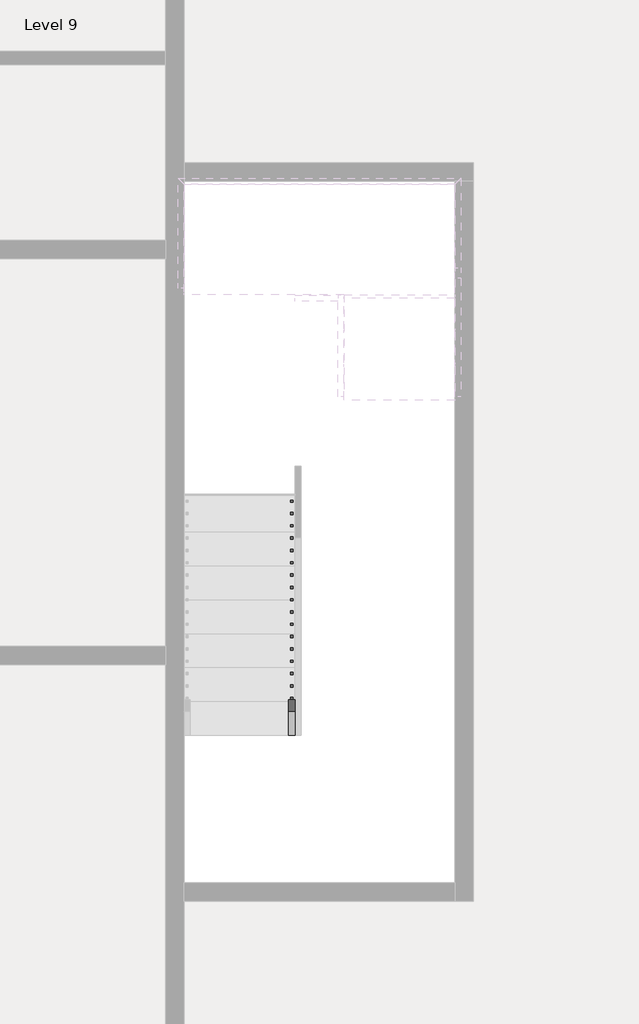
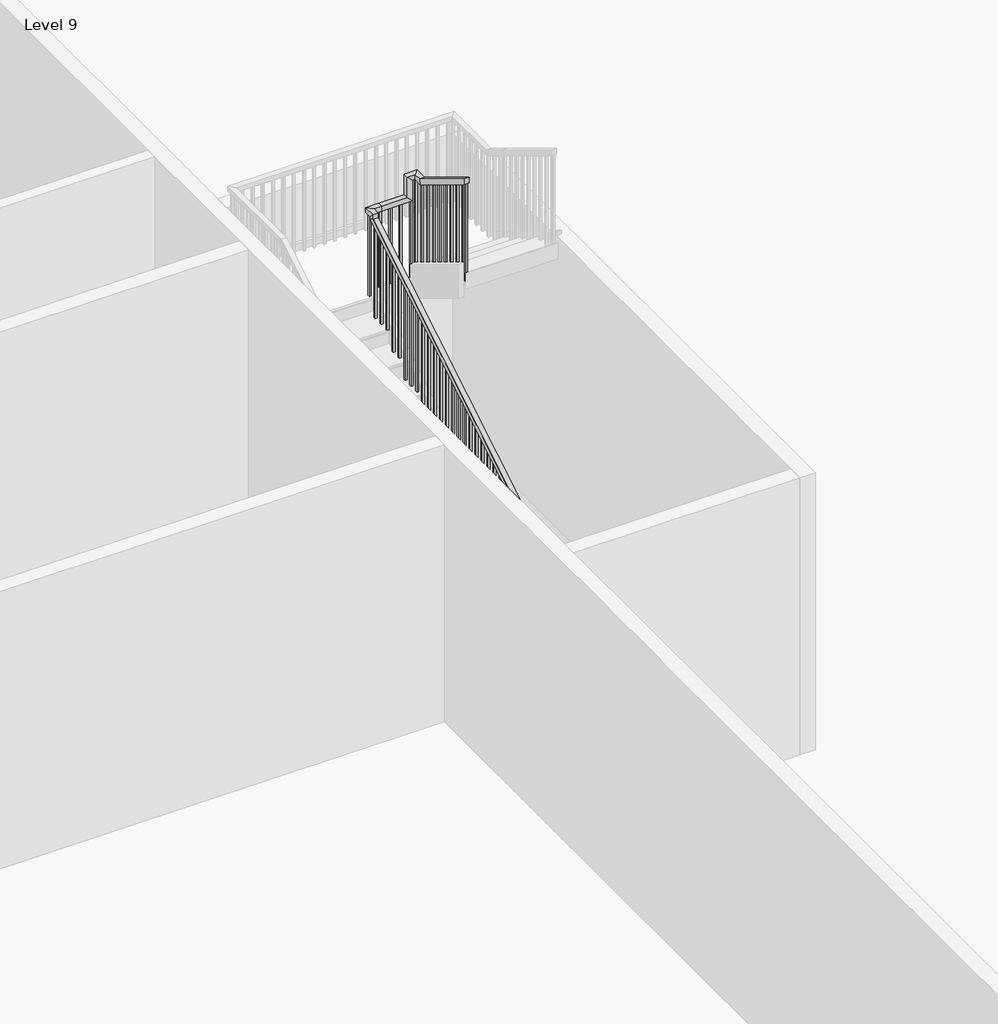
# One storey, part 5 of 8: 1 railing.
"""IFC4 building model written with IfcOpenShell, lengths in millimetres."""

from ifc_helpers import new_model, si_unit, frame, origin, place, context, project, spatial, polyline, outline, extrude, faceted_brep, element, save

model = new_model("IFC4")

# Units and contexts
model_context = context("Model", 3, world=origin())
ifc_project = project(units=[si_unit("LENGTHUNIT", "METRE", prefix="MILLI")], contexts=[model_context])

# Site, building, storey
site = spatial("IfcSite", under=ifc_project)
building = spatial("IfcBuilding", under=site)
storey = spatial("IfcBuildingStorey", under=building, Name="Level 9", Elevation=49618.6172466)

# Railing
placement = place(None, origin())
element("IfcRailing", 1, ObjectType="Handrail - Rectangular", at=placement, inside=storey, context=model_context, shape_type="SolidModel", body=[
    faceted_brep([(-2753.8415084, -23154.3851539, 50702.3505799), (-2753.8415084, -23154.3851539, 50642.9491197), (-2703.0415084, -23154.3851539, 50642.9491197), (-2703.0415084, -23154.3851539, 50702.3505799), (-2753.8415084, -19598.3851539, 52857.5020951), (-2753.8415084, -19547.5851539, 52828.8885136), (-2703.0415084, -19547.5851539, 52828.8885136), (-2703.0415084, -19598.3851539, 52857.5020951), (-2753.8415084, -19598.3851539, 52903.6839133), (-2753.8415084, -19547.5851539, 52852.8839133), (-2703.0415084, -19547.5851539, 52852.8839133), (-2703.0415084, -19598.3851539, 52903.6839133), (-2753.8415084, -19471.3851539, 52903.6839133), (-2753.8415084, -19471.3851539, 52852.8839133), (-2703.0415084, -19522.1851539, 52852.8839133), (-2703.0415084, -19522.1851539, 52903.6839133), (-2626.8415084, -19471.3851539, 52903.6839133), (-2626.8415084, -19471.3851539, 52852.8839133), (-2626.8415084, -19522.1851539, 52852.8839133), (-2626.8415084, -19522.1851539, 52903.6839133), (-2372.8415084, -19471.3851539, 52903.6839133), (-2322.0415084, -19471.3851539, 52852.8839133), (-2322.0415084, -19522.1851539, 52852.8839133), (-2372.8415084, -19522.1851539, 52903.6839133), (-2372.8415084, -19471.3851539, 53119.1990648), (-2322.0415084, -19471.3851539, 53068.3990648), (-2322.0415084, -19522.1851539, 53068.3990648), (-2372.8415084, -19522.1851539, 53119.1990648), (-2245.8415084, -19471.3851539, 53119.1990648), (-2245.8415084, -19471.3851539, 53068.3990648), (-2296.6415084, -19522.1851539, 53068.3990648), (-2296.6415084, -19522.1851539, 53119.1990648), (-2245.8415084, -19598.3851539, 53119.1990648), (-2245.8415084, -19612.5775633, 53068.3990648), (-2296.6415084, -19612.5775633, 53068.3990648), (-2296.6415084, -19598.3851539, 53119.1990648), (-2245.8415084, -20360.3851539, 53581.0172466), (-2296.6415084, -20360.3851539, 53581.0172466), (-2296.6415084, -20360.3851539, 53521.6157863), (-2245.8415084, -20360.3851539, 53521.6157863)], [[[0, 1, 2, 3]], [[1, 0, 4, 5]], [[2, 1, 5, 6]], [[3, 2, 6, 7]], [[0, 3, 7, 4]], [[5, 4, 8, 9]], [[6, 5, 9, 10]], [[7, 6, 10, 11]], [[4, 7, 11, 8]], [[9, 8, 12, 13]], [[10, 9, 13, 14]], [[11, 10, 14, 15]], [[8, 11, 15, 12]], [[13, 12, 16, 17]], [[14, 13, 17, 18]], [[15, 14, 18, 19]], [[12, 15, 19, 16]], [[17, 16, 20, 21]], [[18, 17, 21, 22]], [[19, 18, 22, 23]], [[16, 19, 23, 20]], [[21, 20, 24, 25]], [[22, 21, 25, 26]], [[23, 22, 26, 27]], [[20, 23, 27, 24]], [[25, 24, 28, 29]], [[26, 25, 29, 30]], [[27, 26, 30, 31]], [[24, 27, 31, 28]], [[29, 28, 32, 33]], [[30, 29, 33, 34]], [[31, 30, 34, 35]], [[28, 31, 35, 32]], [[36, 37, 38, 39]], [[33, 32, 36, 39]], [[34, 33, 39, 38]], [[35, 34, 38, 37]], [[32, 35, 37, 36]]]),
    extrude(outline(polyline([(-20319.1101539, 53496.6006348), (-20300.0601539, 53485.0551803), (-20300.0601539, 52497.2839133), (-20319.1101539, 52497.2839133), (-20319.1101539, 53496.6006348)])), frame((-2280.7665084, 0.0, 0.0), z_axis=(1.0, 0.0, 0.0), x_axis=(0.0, 1.0, 0.0)), (0.0, 0.0, 1.0), 19.05),
    extrude(outline(polyline([(-20217.5101539, 53435.0248773), (-20198.4601539, 53423.4794227), (-20198.4601539, 52497.2839133), (-20217.5101539, 52497.2839133), (-20217.5101539, 53435.0248773)])), frame((-2280.7665084, 0.0, 0.0), z_axis=(1.0, 0.0, 0.0), x_axis=(0.0, 1.0, 0.0)), (0.0, 0.0, 1.0), 19.05),
    extrude(outline(polyline([(-20115.9101539, 53373.4491197), (-20096.8601539, 53361.9036651), (-20096.8601539, 52497.2839133), (-20115.9101539, 52497.2839133), (-20115.9101539, 53373.4491197)])), frame((-2280.7665084, 0.0, 0.0), z_axis=(1.0, 0.0, 0.0), x_axis=(0.0, 1.0, 0.0)), (0.0, 0.0, 1.0), 19.05),
    extrude(outline(polyline([(-20014.3101539, 53311.8733621), (-19995.2601539, 53300.3279076), (-19995.2601539, 52327.9505799), (-20014.3101539, 52327.9505799), (-20014.3101539, 53311.8733621)])), frame((-2280.7665084, 0.0, 0.0), z_axis=(1.0, 0.0, 0.0), x_axis=(0.0, 1.0, 0.0)), (0.0, 0.0, 1.0), 19.05),
    extrude(outline(polyline([(-19912.7101539, 53250.2976045), (-19893.6601539, 53238.75215), (-19893.6601539, 52327.9505799), (-19912.7101539, 52327.9505799), (-19912.7101539, 53250.2976045)])), frame((-2280.7665084, 0.0, 0.0), z_axis=(1.0, 0.0, 0.0), x_axis=(0.0, 1.0, 0.0)), (0.0, 0.0, 1.0), 19.05),
    extrude(outline(polyline([(-19811.1101539, 53188.721847), (-19792.0601539, 53177.1763924), (-19792.0601539, 52327.9505799), (-19811.1101539, 52327.9505799), (-19811.1101539, 53188.721847)])), frame((-2280.7665084, 0.0, 0.0), z_axis=(1.0, 0.0, 0.0), x_axis=(0.0, 1.0, 0.0)), (0.0, 0.0, 1.0), 19.05),
    extrude(outline(polyline([(-19709.5101539, 53127.1460894), (-19690.4601539, 53115.6006348), (-19690.4601539, 52158.6172466), (-19709.5101539, 52158.6172466), (-19709.5101539, 53127.1460894)])), frame((-2280.7665084, 0.0, 0.0), z_axis=(1.0, 0.0, 0.0), x_axis=(0.0, 1.0, 0.0)), (0.0, 0.0, 1.0), 19.05),
    extrude(outline(polyline([(-19607.9101539, 53065.5703318), (-19588.8601539, 53054.0248773), (-19588.8601539, 52158.6172466), (-19607.9101539, 52158.6172466), (-19607.9101539, 53065.5703318)])), frame((-2280.7665084, 0.0, 0.0), z_axis=(1.0, 0.0, 0.0), x_axis=(0.0, 1.0, 0.0)), (0.0, 0.0, 1.0), 19.05),
    extrude(outline(polyline([(-2331.5665084, -19506.3101539), (-2331.5665084, -19487.2601539), (-2312.5165084, -19487.2601539), (-2312.5165084, -19506.3101539), (-2331.5665084, -19506.3101539)])), frame((0.0, 0.0, 51989.2839133), z_axis=(0.0, 0.0, 1.0), x_axis=(1.0, 0.0, 0.0)), (0.0, 0.0, 1.0), 1079.1151515),
    extrude(outline(polyline([(-2433.1665084, -19506.3101539), (-2433.1665084, -19487.2601539), (-2414.1165084, -19487.2601539), (-2414.1165084, -19506.3101539), (-2433.1665084, -19506.3101539)])), frame((0.0, 0.0, 51989.2839133), z_axis=(0.0, 0.0, 1.0), x_axis=(1.0, 0.0, 0.0)), (0.0, 0.0, 1.0), 863.6),
    extrude(outline(polyline([(-2534.7665084, -19506.3101539), (-2534.7665084, -19487.2601539), (-2515.7165084, -19487.2601539), (-2515.7165084, -19506.3101539), (-2534.7665084, -19506.3101539)])), frame((0.0, 0.0, 51989.2839133), z_axis=(0.0, 0.0, 1.0), x_axis=(1.0, 0.0, 0.0)), (0.0, 0.0, 1.0), 863.6),
    extrude(outline(polyline([(-2636.3665084, -19506.3101539), (-2636.3665084, -19487.2601539), (-2617.3165084, -19487.2601539), (-2617.3165084, -19506.3101539), (-2636.3665084, -19506.3101539)])), frame((0.0, 0.0, 51989.2839133), z_axis=(0.0, 0.0, 1.0), x_axis=(1.0, 0.0, 0.0)), (0.0, 0.0, 1.0), 863.6),
    extrude(outline(polyline([(-19607.9101539, 52792.3279076), (-19588.8601539, 52803.8733621), (-19588.8601539, 51819.9505799), (-19607.9101539, 51819.9505799), (-19607.9101539, 52792.3279076)])), frame((-2737.9665084, 0.0, 0.0), z_axis=(1.0, 0.0, 0.0), x_axis=(0.0, 1.0, 0.0)), (0.0, 0.0, 1.0), 19.05),
    extrude(outline(polyline([(-19709.5101539, 52730.75215), (-19690.4601539, 52742.2976045), (-19690.4601539, 51819.9505799), (-19709.5101539, 51819.9505799), (-19709.5101539, 52730.75215)])), frame((-2737.9665084, 0.0, 0.0), z_axis=(1.0, 0.0, 0.0), x_axis=(0.0, 1.0, 0.0)), (0.0, 0.0, 1.0), 19.05),
    extrude(outline(polyline([(-19811.1101539, 52669.1763924), (-19792.0601539, 52680.721847), (-19792.0601539, 51819.9505799), (-19811.1101539, 51819.9505799), (-19811.1101539, 52669.1763924)])), frame((-2737.9665084, 0.0, 0.0), z_axis=(1.0, 0.0, 0.0), x_axis=(0.0, 1.0, 0.0)), (0.0, 0.0, 1.0), 19.05),
    extrude(outline(polyline([(-19912.7101539, 52607.6006348), (-19893.6601539, 52619.1460894), (-19893.6601539, 51650.6172466), (-19912.7101539, 51650.6172466), (-19912.7101539, 52607.6006348)])), frame((-2737.9665084, 0.0, 0.0), z_axis=(1.0, 0.0, 0.0), x_axis=(0.0, 1.0, 0.0)), (0.0, 0.0, 1.0), 19.05),
    extrude(outline(polyline([(-20014.3101539, 52546.0248773), (-19995.2601539, 52557.5703318), (-19995.2601539, 51650.6172466), (-20014.3101539, 51650.6172466), (-20014.3101539, 52546.0248773)])), frame((-2737.9665084, 0.0, 0.0), z_axis=(1.0, 0.0, 0.0), x_axis=(0.0, 1.0, 0.0)), (0.0, 0.0, 1.0), 19.05),
    extrude(outline(polyline([(-20115.9101539, 52484.4491197), (-20096.8601539, 52495.9945742), (-20096.8601539, 51481.2839133), (-20115.9101539, 51481.2839133), (-20115.9101539, 52484.4491197)])), frame((-2737.9665084, 0.0, 0.0), z_axis=(1.0, 0.0, 0.0), x_axis=(0.0, 1.0, 0.0)), (0.0, 0.0, 1.0), 19.05),
    extrude(outline(polyline([(-20217.5101539, 52422.8733621), (-20198.4601539, 52434.4188166), (-20198.4601539, 51481.2839133), (-20217.5101539, 51481.2839133), (-20217.5101539, 52422.8733621)])), frame((-2737.9665084, 0.0, 0.0), z_axis=(1.0, 0.0, 0.0), x_axis=(0.0, 1.0, 0.0)), (0.0, 0.0, 1.0), 19.05),
    extrude(outline(polyline([(-20319.1101539, 52361.2976045), (-20300.0601539, 52372.8430591), (-20300.0601539, 51481.2839133), (-20319.1101539, 51481.2839133), (-20319.1101539, 52361.2976045)])), frame((-2737.9665084, 0.0, 0.0), z_axis=(1.0, 0.0, 0.0), x_axis=(0.0, 1.0, 0.0)), (0.0, 0.0, 1.0), 19.05),
    extrude(outline(polyline([(-20420.7101539, 52299.721847), (-20401.6601539, 52311.2673015), (-20401.6601539, 51311.9505799), (-20420.7101539, 51311.9505799), (-20420.7101539, 52299.721847)])), frame((-2737.9665084, 0.0, 0.0), z_axis=(1.0, 0.0, 0.0), x_axis=(0.0, 1.0, 0.0)), (0.0, 0.0, 1.0), 19.05),
    extrude(outline(polyline([(-20522.3101539, 52238.1460894), (-20503.2601539, 52249.6915439), (-20503.2601539, 51311.9505799), (-20522.3101539, 51311.9505799), (-20522.3101539, 52238.1460894)])), frame((-2737.9665084, 0.0, 0.0), z_axis=(1.0, 0.0, 0.0), x_axis=(0.0, 1.0, 0.0)), (0.0, 0.0, 1.0), 19.05),
    extrude(outline(polyline([(-20623.9101539, 52176.5703318), (-20604.8601539, 52188.1157863), (-20604.8601539, 51311.9505799), (-20623.9101539, 51311.9505799), (-20623.9101539, 52176.5703318)])), frame((-2737.9665084, 0.0, 0.0), z_axis=(1.0, 0.0, 0.0), x_axis=(0.0, 1.0, 0.0)), (0.0, 0.0, 1.0), 19.05),
    extrude(outline(polyline([(-20725.5101539, 52114.9945742), (-20706.4601539, 52126.5400288), (-20706.4601539, 51142.6172466), (-20725.5101539, 51142.6172466), (-20725.5101539, 52114.9945742)])), frame((-2737.9665084, 0.0, 0.0), z_axis=(1.0, 0.0, 0.0), x_axis=(0.0, 1.0, 0.0)), (0.0, 0.0, 1.0), 19.05),
    extrude(outline(polyline([(-20827.1101539, 52053.4188166), (-20808.0601539, 52064.9642712), (-20808.0601539, 51142.6172466), (-20827.1101539, 51142.6172466), (-20827.1101539, 52053.4188166)])), frame((-2737.9665084, 0.0, 0.0), z_axis=(1.0, 0.0, 0.0), x_axis=(0.0, 1.0, 0.0)), (0.0, 0.0, 1.0), 19.05),
    extrude(outline(polyline([(-20928.7101539, 51991.8430591), (-20909.6601539, 52003.3885136), (-20909.6601539, 51142.6172466), (-20928.7101539, 51142.6172466), (-20928.7101539, 51991.8430591)])), frame((-2737.9665084, 0.0, 0.0), z_axis=(1.0, 0.0, 0.0), x_axis=(0.0, 1.0, 0.0)), (0.0, 0.0, 1.0), 19.05),
    extrude(outline(polyline([(-21030.3101539, 51930.2673015), (-21011.2601539, 51941.812756), (-21011.2601539, 50973.2839133), (-21030.3101539, 50973.2839133), (-21030.3101539, 51930.2673015)])), frame((-2737.9665084, 0.0, 0.0), z_axis=(1.0, 0.0, 0.0), x_axis=(0.0, 1.0, 0.0)), (0.0, 0.0, 1.0), 19.05),
    extrude(outline(polyline([(-21131.9101539, 51868.6915439), (-21112.8601539, 51880.2369985), (-21112.8601539, 50973.2839133), (-21131.9101539, 50973.2839133), (-21131.9101539, 51868.6915439)])), frame((-2737.9665084, 0.0, 0.0), z_axis=(1.0, 0.0, 0.0), x_axis=(0.0, 1.0, 0.0)), (0.0, 0.0, 1.0), 19.05),
    extrude(outline(polyline([(-21233.5101539, 51807.1157863), (-21214.4601539, 51818.6612409), (-21214.4601539, 50803.9505799), (-21233.5101539, 50803.9505799), (-21233.5101539, 51807.1157863)])), frame((-2737.9665084, 0.0, 0.0), z_axis=(1.0, 0.0, 0.0), x_axis=(0.0, 1.0, 0.0)), (0.0, 0.0, 1.0), 19.05),
    extrude(outline(polyline([(-21335.1101539, 51745.5400288), (-21316.0601539, 51757.0854833), (-21316.0601539, 50803.9505799), (-21335.1101539, 50803.9505799), (-21335.1101539, 51745.5400288)])), frame((-2737.9665084, 0.0, 0.0), z_axis=(1.0, 0.0, 0.0), x_axis=(0.0, 1.0, 0.0)), (0.0, 0.0, 1.0), 19.05),
    extrude(outline(polyline([(-21436.7101539, 51683.9642712), (-21417.6601539, 51695.5097257), (-21417.6601539, 50803.9505799), (-21436.7101539, 50803.9505799), (-21436.7101539, 51683.9642712)])), frame((-2737.9665084, 0.0, 0.0), z_axis=(1.0, 0.0, 0.0), x_axis=(0.0, 1.0, 0.0)), (0.0, 0.0, 1.0), 19.05),
    extrude(outline(polyline([(-21538.3101539, 51622.3885136), (-21519.2601539, 51633.9339682), (-21519.2601539, 50634.6172466), (-21538.3101539, 50634.6172466), (-21538.3101539, 51622.3885136)])), frame((-2737.9665084, 0.0, 0.0), z_axis=(1.0, 0.0, 0.0), x_axis=(0.0, 1.0, 0.0)), (0.0, 0.0, 1.0), 19.05),
    extrude(outline(polyline([(-21639.9101539, 51560.812756), (-21620.8601539, 51572.3582106), (-21620.8601539, 50634.6172466), (-21639.9101539, 50634.6172466), (-21639.9101539, 51560.812756)])), frame((-2737.9665084, 0.0, 0.0), z_axis=(1.0, 0.0, 0.0), x_axis=(0.0, 1.0, 0.0)), (0.0, 0.0, 1.0), 19.05),
    extrude(outline(polyline([(-21741.5101539, 51499.2369985), (-21722.4601539, 51510.782453), (-21722.4601539, 50634.6172466), (-21741.5101539, 50634.6172466), (-21741.5101539, 51499.2369985)])), frame((-2737.9665084, 0.0, 0.0), z_axis=(1.0, 0.0, 0.0), x_axis=(0.0, 1.0, 0.0)), (0.0, 0.0, 1.0), 19.05),
    extrude(outline(polyline([(-21843.1101539, 51437.6612409), (-21824.0601539, 51449.2066954), (-21824.0601539, 50465.2839133), (-21843.1101539, 50465.2839133), (-21843.1101539, 51437.6612409)])), frame((-2737.9665084, 0.0, 0.0), z_axis=(1.0, 0.0, 0.0), x_axis=(0.0, 1.0, 0.0)), (0.0, 0.0, 1.0), 19.05),
    extrude(outline(polyline([(-21944.7101539, 51376.0854833), (-21925.6601539, 51387.6309379), (-21925.6601539, 50465.2839133), (-21944.7101539, 50465.2839133), (-21944.7101539, 51376.0854833)])), frame((-2737.9665084, 0.0, 0.0), z_axis=(1.0, 0.0, 0.0), x_axis=(0.0, 1.0, 0.0)), (0.0, 0.0, 1.0), 19.05),
    extrude(outline(polyline([(-22046.3101539, 51314.5097257), (-22027.2601539, 51326.0551803), (-22027.2601539, 50465.2839133), (-22046.3101539, 50465.2839133), (-22046.3101539, 51314.5097257)])), frame((-2737.9665084, 0.0, 0.0), z_axis=(1.0, 0.0, 0.0), x_axis=(0.0, 1.0, 0.0)), (0.0, 0.0, 1.0), 19.05),
    extrude(outline(polyline([(-22147.9101539, 51252.9339682), (-22128.8601539, 51264.4794227), (-22128.8601539, 50295.9505799), (-22147.9101539, 50295.9505799), (-22147.9101539, 51252.9339682)])), frame((-2737.9665084, 0.0, 0.0), z_axis=(1.0, 0.0, 0.0), x_axis=(0.0, 1.0, 0.0)), (0.0, 0.0, 1.0), 19.05),
    extrude(outline(polyline([(-22249.5101539, 51191.3582106), (-22230.4601539, 51202.9036651), (-22230.4601539, 50295.9505799), (-22249.5101539, 50295.9505799), (-22249.5101539, 51191.3582106)])), frame((-2737.9665084, 0.0, 0.0), z_axis=(1.0, 0.0, 0.0), x_axis=(0.0, 1.0, 0.0)), (0.0, 0.0, 1.0), 19.05),
    extrude(outline(polyline([(-22351.1101539, 51129.782453), (-22332.0601539, 51141.3279076), (-22332.0601539, 50126.6172466), (-22351.1101539, 50126.6172466), (-22351.1101539, 51129.782453)])), frame((-2737.9665084, 0.0, 0.0), z_axis=(1.0, 0.0, 0.0), x_axis=(0.0, 1.0, 0.0)), (0.0, 0.0, 1.0), 19.05),
    extrude(outline(polyline([(-22452.7101539, 51068.2066954), (-22433.6601539, 51079.75215), (-22433.6601539, 50126.6172466), (-22452.7101539, 50126.6172466), (-22452.7101539, 51068.2066954)])), frame((-2737.9665084, 0.0, 0.0), z_axis=(1.0, 0.0, 0.0), x_axis=(0.0, 1.0, 0.0)), (0.0, 0.0, 1.0), 19.05),
    extrude(outline(polyline([(-22554.3101539, 51006.6309379), (-22535.2601539, 51018.1763924), (-22535.2601539, 50126.6172466), (-22554.3101539, 50126.6172466), (-22554.3101539, 51006.6309379)])), frame((-2737.9665084, 0.0, 0.0), z_axis=(1.0, 0.0, 0.0), x_axis=(0.0, 1.0, 0.0)), (0.0, 0.0, 1.0), 19.05),
    extrude(outline(polyline([(-22655.9101539, 50945.0551803), (-22636.8601539, 50956.6006348), (-22636.8601539, 49957.2839133), (-22655.9101539, 49957.2839133), (-22655.9101539, 50945.0551803)])), frame((-2737.9665084, 0.0, 0.0), z_axis=(1.0, 0.0, 0.0), x_axis=(0.0, 1.0, 0.0)), (0.0, 0.0, 1.0), 19.05),
    extrude(outline(polyline([(-22757.5101539, 50883.4794227), (-22738.4601539, 50895.0248773), (-22738.4601539, 49957.2839133), (-22757.5101539, 49957.2839133), (-22757.5101539, 50883.4794227)])), frame((-2737.9665084, 0.0, 0.0), z_axis=(1.0, 0.0, 0.0), x_axis=(0.0, 1.0, 0.0)), (0.0, 0.0, 1.0), 19.05),
    extrude(outline(polyline([(-22859.1101539, 50821.9036651), (-22840.0601539, 50833.4491197), (-22840.0601539, 49957.2839133), (-22859.1101539, 49957.2839133), (-22859.1101539, 50821.9036651)])), frame((-2737.9665084, 0.0, 0.0), z_axis=(1.0, 0.0, 0.0), x_axis=(0.0, 1.0, 0.0)), (0.0, 0.0, 1.0), 19.05),
    extrude(outline(polyline([(-22960.7101539, 50760.3279076), (-22941.6601539, 50771.8733621), (-22941.6601539, 49787.9505799), (-22960.7101539, 49787.9505799), (-22960.7101539, 50760.3279076)])), frame((-2737.9665084, 0.0, 0.0), z_axis=(1.0, 0.0, 0.0), x_axis=(0.0, 1.0, 0.0)), (0.0, 0.0, 1.0), 19.05),
    extrude(outline(polyline([(-23062.3101539, 50698.75215), (-23043.2601539, 50710.2976045), (-23043.2601539, 49787.9505799), (-23062.3101539, 49787.9505799), (-23062.3101539, 50698.75215)])), frame((-2737.9665084, 0.0, 0.0), z_axis=(1.0, 0.0, 0.0), x_axis=(0.0, 1.0, 0.0)), (0.0, 0.0, 1.0), 19.05),
    extrude(outline(polyline([(-2280.7665084, -19506.3101539), (-2280.7665084, -19487.2601539), (-2261.7165084, -19487.2601539), (-2261.7165084, -19506.3101539), (-2280.7665084, -19506.3101539)])), frame((0.0, 0.0, 51989.2839133), z_axis=(0.0, 0.0, 1.0), x_axis=(1.0, 0.0, 0.0)), (0.0, 0.0, 1.0), 1079.1151515),
    extrude(outline(polyline([(-2718.9165084, -19506.3101539), (-2737.9665084, -19506.3101539), (-2737.9665084, -19487.2601539), (-2718.9165084, -19487.2601539), (-2718.9165084, -19506.3101539)])), frame((0.0, 0.0, 51989.2839133), z_axis=(0.0, 0.0, 1.0), x_axis=(1.0, 0.0, 0.0)), (0.0, 0.0, 1.0), 863.6),
    extrude(outline(polyline([(-20360.3851539, 53521.6157863), (-20341.3351539, 53510.0703318), (-20341.3351539, 52497.2839133), (-20360.3851539, 52497.2839133), (-20360.3851539, 53521.6157863)])), frame((-2280.7665084, 0.0, 0.0), z_axis=(1.0, 0.0, 0.0), x_axis=(0.0, 1.0, 0.0)), (0.0, 0.0, 1.0), 19.05),
    extrude(outline(polyline([(-23154.3851539, 50642.9491197), (-23135.3351539, 50654.4945742), (-23135.3351539, 49787.9505799), (-23154.3851539, 49787.9505799), (-23154.3851539, 50642.9491197)])), frame((-2737.9665084, 0.0, 0.0), z_axis=(1.0, 0.0, 0.0), x_axis=(0.0, 1.0, 0.0)), (0.0, 0.0, 1.0), 19.05),
])

save(model, "model.ifc")

# Revit data of these elements
# Type "Handrail - Rectangular"
#   Assembly Code = "C2010400"
#   built-in parameter 1008612 = 0.0416667 (stored number, unit not read)
#   built-in parameter 1008611 = 0.0416667 (stored number, unit not read)
#   built-in parameter 1008609 = 0.333333 (stored number, unit not read)
#   built-in parameter 1008604 = 0.166667 (stored number, unit not read)
#   built-in parameter 1008603 = 0.166667 (stored number, unit not read)
#   Railing Height = 3' - 0"
#   built-in parameter 1008630 = 2
#   built-in parameter 1008610 = 2
#   built-in parameter 1008618 = Baluster - Square : 3/4"
# Element 1 (IfcRailing, "Handrail - Rectangular")
#   Phase Created = New Construction
